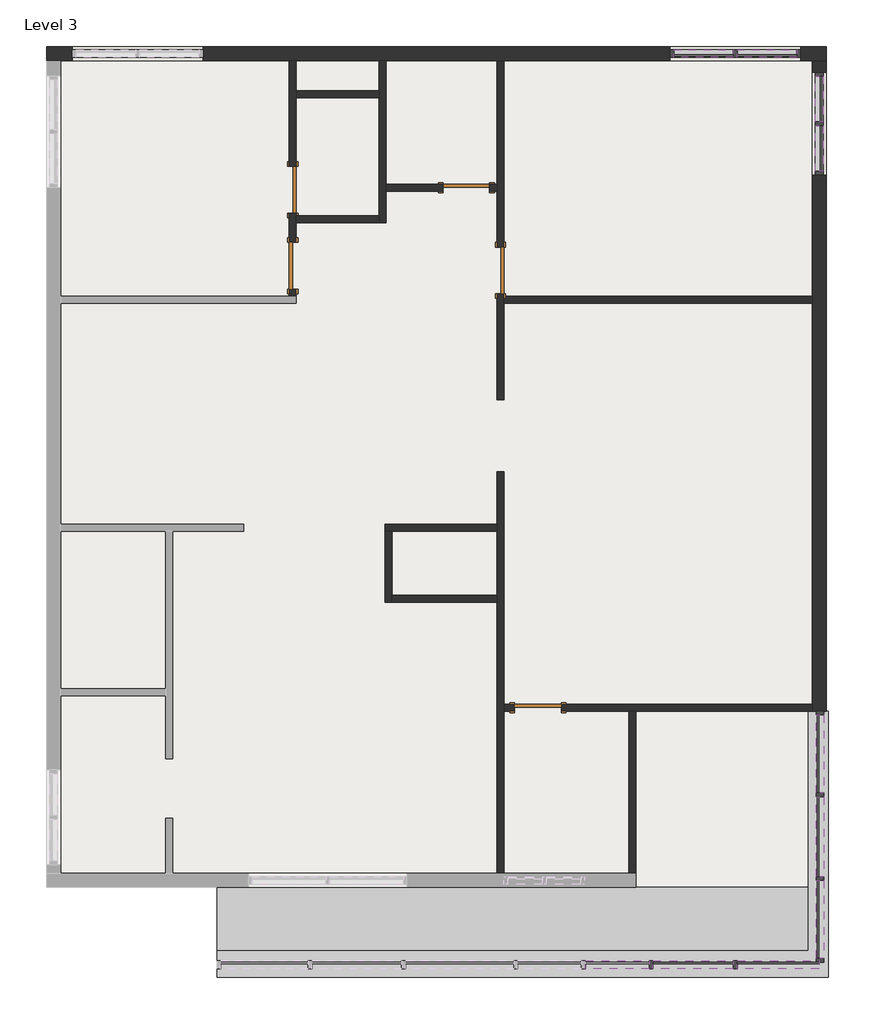
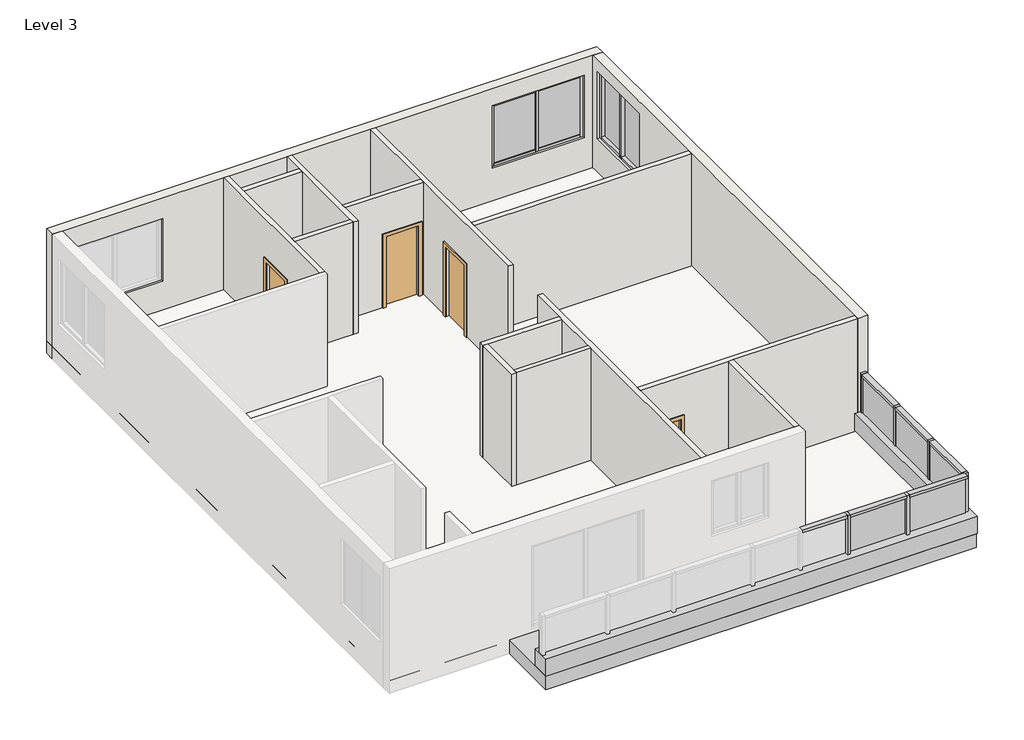
# One storey, part 2 of 2: 26 members, 15 walls, 9 plates, 5 doors, 1 proxy, 1 roof.
"""IFC4 building model written with IfcOpenShell, lengths in millimetres."""

from ifc_helpers import new_model, si_unit, frame, origin, place, context, project, spatial, polyline, outline, extrude, faceted_brep, transform, mapped, element, save
from components import generic_models_5_generic_models_5_36a2ceba, door_f2b275c1, door_d8f5dbb5, member_3a0a7659, member_801a2072, member_0bc49b9d, member_ce46b7cd, member_bcb10b1d, member_032a0f9a, member_dda01c07, member_04769ced, member_d37749d9, member_69204bcc, member_aead4eab, member_d6537dc6, member_1988c634, member_477baa08, system_panel_glazed_822919b4, system_panel_glazed_5228c6df, system_panel_glazed_6547e81a, system_panel_glazed_b56c0438, system_panel_glazed_688ed8e9, system_panel_glazed_5ee7ee01

model = new_model("IFC4")

# Units and contexts
model_context = context("Model", 3, world=origin())
ifc_project = project(units=[si_unit("LENGTHUNIT", "METRE", prefix="MILLI")], contexts=[model_context])

# Site, building, storey
site = spatial("IfcSite", under=ifc_project)
building = spatial("IfcBuilding", under=site)
storey = spatial("IfcBuildingStorey", under=building, Name="Level 3", Elevation=6096.0)

# Proxy
placement = place(None, origin())
generic_models_5_generic_models_5_shape = generic_models_5_generic_models_5_36a2ceba(model_context)
element("IfcBuildingElementProxy", 1, Name="Generic Models 5 : Generic Models 5", ObjectType="Generic Models 5 : Generic Models 5", at=placement, inside=storey, context=model_context, shape_type="MappedRepresentation", body=[
    mapped(generic_models_5_generic_models_5_shape, transform((0.0, 0.0, 0.0), x_axis=(1.0, 0.0, 0.0), y_axis=(0.0, 1.0, 0.0), z_axis=(0.0, 0.0, 1.0))),
])

# Doors
door_shape = door_f2b275c1(model_context)
element("IfcDoor", 2, ObjectType="Single-Flush : 30\" x 80\"", at=placement, inside=storey, context=model_context, shape_type="MappedRepresentation", body=[
    mapped(door_shape, transform((-14978.0695233, -3993.8252569, 6096.0), x_axis=(0.0, -1.0, 0.0), y_axis=(1.0, 0.0, 0.0), z_axis=(0.0, 0.0, 1.0))),
])
element("IfcDoor", 3, ObjectType="Single-Flush : 30\" x 80\"", at=placement, inside=storey, context=model_context, shape_type="MappedRepresentation", body=[
    mapped(door_shape, transform((-10977.5695233, -11201.0752569, 6096.0), x_axis=(-1.0, 0.0, 0.0), y_axis=(0.0, -1.0, 0.0), z_axis=(0.0, 0.0, 1.0))),
])
door_2_shape = door_d8f5dbb5(model_context)
element("IfcDoor", 4, ObjectType="Single-Flush : 30\" x 80\"", at=placement, inside=storey, context=model_context, shape_type="MappedRepresentation", body=[
    mapped(door_2_shape, transform((-14978.0695233, -2755.5752569, 6096.0), x_axis=(0.0, -1.0, 0.0), y_axis=(1.0, 0.0, 0.0), z_axis=(0.0, 0.0, 1.0))),
])
element("IfcDoor", 5, ObjectType="Single-Flush : 30\" x 80\"", at=placement, inside=storey, context=model_context, shape_type="MappedRepresentation", body=[
    mapped(door_2_shape, transform((-12145.9695233, -2723.8252569, 6096.0), x_axis=(1.0, 0.0, 0.0), y_axis=(0.0, 1.0, 0.0), z_axis=(0.0, 0.0, 1.0))),
])
element("IfcDoor", 6, ObjectType="Single-Flush : 30\" x 80\"", at=placement, inside=storey, context=model_context, shape_type="MappedRepresentation", body=[
    mapped(door_2_shape, transform((-11587.1695233, -4070.0252569, 6096.0), x_axis=(0.0, -1.0, 0.0), y_axis=(1.0, 0.0, 0.0), z_axis=(0.0, 0.0, 1.0))),
])

# Members
member_shape = member_3a0a7659(model_context)
element("IfcMember", 7, ObjectType="Rectangular Mullion : 2.5\" x 5\" rectangular", at=placement, inside=storey, context=model_context, shape_type="MappedRepresentation", body=[
    mapped(member_shape, transform((-6386.5195233, -1644.3252569, 8857.8668559), x_axis=(0.0, 0.0, 1.0), y_axis=(-1.0, 0.0, 0.0), z_axis=(0.0, -1.0, 0.0))),
])
element("IfcMember", 8, ObjectType="Rectangular Mullion : 2.5\" x 5\" rectangular", at=placement, inside=storey, context=model_context, shape_type="MappedRepresentation", body=[
    mapped(member_shape, transform((-6386.5195233, -2450.7752569, 8857.8668559), x_axis=(0.0, 0.0, 1.0), y_axis=(-1.0, 0.0, 0.0), z_axis=(0.0, -1.0, 0.0))),
])
element("IfcMember", 9, ObjectType="Rectangular Mullion : 2.5\" x 5\" rectangular", at=placement, inside=storey, context=model_context, shape_type="MappedRepresentation", body=[
    mapped(member_shape, transform((-6386.5195233, -1707.8252569, 7223.9300621), x_axis=(0.0, 0.0, -1.0), y_axis=(-1.0, 0.0, 0.0), z_axis=(0.0, 1.0, 0.0))),
])
element("IfcMember", 10, ObjectType="Rectangular Mullion : 2.5\" x 5\" rectangular", at=placement, inside=storey, context=model_context, shape_type="MappedRepresentation", body=[
    mapped(member_shape, transform((-6386.5195233, -901.3752569, 7223.9300621), x_axis=(0.0, 0.0, -1.0), y_axis=(-1.0, 0.0, 0.0), z_axis=(0.0, 1.0, 0.0))),
])
member_2_shape = member_801a2072(model_context)
element("IfcMember", 11, ObjectType="Rectangular Mullion : 2.5\" x 5\" rectangular", at=placement, inside=storey, context=model_context, shape_type="MappedRepresentation", body=[
    mapped(member_2_shape, transform((-8761.4195233, -533.0752569, 8728.0505251), x_axis=(0.0, 0.0, 1.0), y_axis=(0.0, 1.0, 0.0), z_axis=(-1.0, 0.0, 0.0))),
])
element("IfcMember", 12, ObjectType="Rectangular Mullion : 2.5\" x 5\" rectangular", at=placement, inside=storey, context=model_context, shape_type="MappedRepresentation", body=[
    mapped(member_2_shape, transform((-7726.3695233, -533.0752569, 8728.0505251), x_axis=(0.0, 0.0, 1.0), y_axis=(0.0, 1.0, 0.0), z_axis=(-1.0, 0.0, 0.0))),
])
element("IfcMember", 13, ObjectType="Rectangular Mullion : 2.5\" x 5\" rectangular", at=placement, inside=storey, context=model_context, shape_type="MappedRepresentation", body=[
    mapped(member_2_shape, transform((-6754.8195233, -533.0752569, 7198.162091), x_axis=(0.0, 0.0, -1.0), y_axis=(0.0, 1.0, 0.0), z_axis=(1.0, 0.0, 0.0))),
])
element("IfcMember", 14, ObjectType="Rectangular Mullion : 2.5\" x 5\" rectangular", at=placement, inside=storey, context=model_context, shape_type="MappedRepresentation", body=[
    mapped(member_2_shape, transform((-7789.8695233, -533.0752569, 7198.162091), x_axis=(0.0, 0.0, -1.0), y_axis=(0.0, 1.0, 0.0), z_axis=(1.0, 0.0, 0.0))),
])
member_3_shape = member_0bc49b9d(model_context)
element("IfcMember", 15, ObjectType="Rectangular Mullion : 2.5\" x 5\" rectangular", at=placement, inside=storey, context=model_context, shape_type="MappedRepresentation", body=[
    mapped(member_3_shape, transform((-6386.5195233, -1676.0752569, 7223.9300621), x_axis=(0.0, -1.0, 0.0), y_axis=(-1.0, 0.0, 0.0), z_axis=(0.0, 0.0, -1.0))),
])
member_4_shape = member_ce46b7cd(model_context)
element("IfcMember", 16, ObjectType="Rectangular Mullion : 2.5\" x 5\" rectangular", at=placement, inside=storey, context=model_context, shape_type="MappedRepresentation", body=[
    mapped(member_4_shape, transform((-6386.5195233, -837.8752569, 8857.8668559), x_axis=(0.0, 1.0, 0.0), y_axis=(-1.0, 0.0, 0.0), z_axis=(0.0, 0.0, 1.0))),
])
element("IfcMember", 17, ObjectType="Rectangular Mullion : 2.5\" x 5\" rectangular", at=placement, inside=storey, context=model_context, shape_type="MappedRepresentation", body=[
    mapped(member_4_shape, transform((-6386.5195233, -2514.2752569, 7223.9300621), x_axis=(0.0, -1.0, 0.0), y_axis=(-1.0, 0.0, 0.0), z_axis=(0.0, 0.0, -1.0))),
])
member_5_shape = member_bcb10b1d(model_context)
element("IfcMember", 18, ObjectType="Rectangular Mullion : 2.5\" x 5\" rectangular", at=placement, inside=storey, context=model_context, shape_type="MappedRepresentation", body=[
    mapped(member_5_shape, transform((-8824.9195233, -533.0752569, 7198.162091), x_axis=(-1.0, 0.0, 0.0), y_axis=(0.0, 1.0, 0.0), z_axis=(0.0, 0.0, -1.0))),
])
element("IfcMember", 19, ObjectType="Rectangular Mullion : 2.5\" x 5\" rectangular", at=placement, inside=storey, context=model_context, shape_type="MappedRepresentation", body=[
    mapped(member_5_shape, transform((-6691.3195233, -533.0752569, 8728.0505251), x_axis=(1.0, 0.0, 0.0), y_axis=(0.0, 1.0, 0.0), z_axis=(0.0, 0.0, 1.0))),
])
member_6_shape = member_032a0f9a(model_context)
element("IfcMember", 20, ObjectType="Rectangular Mullion : 2.5\" x 5\" rectangular", at=placement, inside=storey, context=model_context, shape_type="MappedRepresentation", body=[
    mapped(member_6_shape, transform((-7758.1195233, -533.0752569, 7198.162091), x_axis=(-1.0, 0.0, 0.0), y_axis=(0.0, 1.0, 0.0), z_axis=(0.0, 0.0, -1.0))),
])
member_7_shape = member_dda01c07(model_context)
element("IfcMember", 21, ObjectType="Rectangular Mullion : 2.5\" x 5\" rectangular", at=placement, inside=storey, context=model_context, shape_type="MappedRepresentation", body=[
    mapped(member_7_shape, transform((-9129.7195233, -15398.1130528, 6841.9204311), x_axis=(1.0, 0.0, 0.0), y_axis=(0.0, -1.0, 0.0), z_axis=(0.0, 0.0, -1.0))),
])
element("IfcMember", 22, ObjectType="Rectangular Mullion : 2.5\" x 5\" rectangular", at=placement, inside=storey, context=model_context, shape_type="MappedRepresentation", body=[
    mapped(member_7_shape, transform((-7758.1195233, -15398.1130528, 6841.9204311), x_axis=(1.0, 0.0, 0.0), y_axis=(0.0, -1.0, 0.0), z_axis=(0.0, 0.0, -1.0))),
])
member_8_shape = member_04769ced(model_context)
element("IfcMember", 23, ObjectType="Rectangular Mullion : 2.5\" x 5\" rectangular", at=placement, inside=storey, context=model_context, shape_type="MappedRepresentation", body=[
    mapped(member_8_shape, transform((-9161.4695233, -15398.1130528, 7802.9269124), x_axis=(0.0, 0.0, 1.0), y_axis=(0.0, -1.0, 0.0), z_axis=(1.0, 0.0, 0.0))),
])
member_9_shape = member_d37749d9(model_context)
element("IfcMember", 24, ObjectType="Rectangular Mullion : 2.5\" x 5\" rectangular", at=placement, inside=storey, context=model_context, shape_type="MappedRepresentation", body=[
    mapped(member_9_shape, transform((-7789.8695233, -15398.1130528, 7802.9269124), x_axis=(0.0, 0.0, 1.0), y_axis=(0.0, -1.0, 0.0), z_axis=(1.0, 0.0, 0.0))),
])
member_10_shape = member_69204bcc(model_context)
element("IfcMember", 25, ObjectType="Rectangular Mullion : 2.5\" x 5\" rectangular", at=placement, inside=storey, context=model_context, shape_type="MappedRepresentation", body=[
    mapped(member_10_shape, transform((-6386.5195233, -15398.1130528, 7802.9269124), x_axis=(0.0, 0.0, 1.0), y_axis=(0.0, -1.0, 0.0), z_axis=(1.0, 0.0, 0.0))),
])
member_11_shape = member_aead4eab(model_context)
element("IfcMember", 26, ObjectType="Rectangular Mullion : 2.5\" x 5\" rectangular", at=placement, inside=storey, context=model_context, shape_type="MappedRepresentation", body=[
    mapped(member_11_shape, transform((-6374.7212454, -15353.6630528, 7790.2317703), x_axis=(0.0, -1.0, 0.0), y_axis=(1.0, 0.0, 0.0), z_axis=(0.0, 0.0, 1.0))),
])
member_12_shape = member_d6537dc6(model_context)
element("IfcMember", 27, ObjectType="Rectangular Mullion : 2.5\" x 5\" rectangular", at=placement, inside=storey, context=model_context, shape_type="MappedRepresentation", body=[
    mapped(member_12_shape, transform((-6374.7212454, -14020.2671209, 7790.2317703), x_axis=(0.0, 0.0, 1.0), y_axis=(1.0, 0.0, 0.0), z_axis=(0.0, 1.0, 0.0))),
])
element("IfcMember", 28, ObjectType="Rectangular Mullion : 2.5\" x 5\" rectangular", at=placement, inside=storey, context=model_context, shape_type="MappedRepresentation", body=[
    mapped(member_12_shape, transform((-6374.7212454, -11321.7252569, 7790.2317703), x_axis=(0.0, 0.0, 1.0), y_axis=(1.0, 0.0, 0.0), z_axis=(0.0, 1.0, 0.0))),
])
member_13_shape = member_1988c634(model_context)
element("IfcMember", 29, ObjectType="Rectangular Mullion : 2.5\" x 5\" rectangular", at=placement, inside=storey, context=model_context, shape_type="MappedRepresentation", body=[
    mapped(member_13_shape, transform((-6374.7212454, -13988.5171209, 6841.9204311), x_axis=(0.0, 1.0, 0.0), y_axis=(1.0, 0.0, 0.0), z_axis=(0.0, 0.0, -1.0))),
])
element("IfcMember", 30, ObjectType="Rectangular Mullion : 2.5\" x 5\" rectangular", at=placement, inside=storey, context=model_context, shape_type="MappedRepresentation", body=[
    mapped(member_13_shape, transform((-6374.7212454, -12623.3711889, 6841.9204311), x_axis=(0.0, 1.0, 0.0), y_axis=(1.0, 0.0, 0.0), z_axis=(0.0, 0.0, -1.0))),
])
member_14_shape = member_477baa08(model_context)
element("IfcMember", 31, ObjectType="Rectangular Mullion : 2.5\" x 5\" rectangular", at=placement, inside=storey, context=model_context, shape_type="MappedRepresentation", body=[
    mapped(member_14_shape, transform((-6374.7212454, -12655.1211889, 7790.2317703), x_axis=(0.0, 0.0, 1.0), y_axis=(1.0, 0.0, 0.0), z_axis=(0.0, 1.0, 0.0))),
])
element("IfcMember", 32, ObjectType="Rectangular Mullion : 2.5\" x 5\" rectangular", at=placement, inside=storey, context=model_context, shape_type="MappedRepresentation", body=[
    mapped(member_11_shape, transform((-6374.7212454, -11258.2252569, 6841.9204311), x_axis=(0.0, 1.0, 0.0), y_axis=(1.0, 0.0, 0.0), z_axis=(0.0, 0.0, -1.0))),
])

# Plates
system_panel_glazed_shape = system_panel_glazed_822919b4(model_context)
element("IfcPlate", 33, ObjectType="System Panel : Glazed", at=placement, inside=storey, context=model_context, shape_type="MappedRepresentation", body=[
    mapped(system_panel_glazed_shape, transform((-6386.5195233, -1272.8502569, 7287.4300621), x_axis=(0.0, -1.0, 0.0), y_axis=(1.0, 0.0, 0.0), z_axis=(0.0, 0.0, 1.0))),
])
element("IfcPlate", 34, ObjectType="System Panel : Glazed", at=placement, inside=storey, context=model_context, shape_type="MappedRepresentation", body=[
    mapped(system_panel_glazed_shape, transform((-6386.5195233, -2079.3002569, 7287.4300621), x_axis=(0.0, -1.0, 0.0), y_axis=(1.0, 0.0, 0.0), z_axis=(0.0, 0.0, 1.0))),
])
system_panel_glazed_2_shape = system_panel_glazed_5228c6df(model_context)
element("IfcPlate", 35, ObjectType="System Panel : Glazed", at=placement, inside=storey, context=model_context, shape_type="MappedRepresentation", body=[
    mapped(system_panel_glazed_2_shape, transform((-7240.5945233, -533.0752569, 7261.662091), x_axis=(-1.0, 0.0, 0.0), y_axis=(0.0, -1.0, 0.0), z_axis=(0.0, 0.0, 1.0))),
])
element("IfcPlate", 36, ObjectType="System Panel : Glazed", at=placement, inside=storey, context=model_context, shape_type="MappedRepresentation", body=[
    mapped(system_panel_glazed_2_shape, transform((-8275.6445233, -533.0752569, 7261.662091), x_axis=(-1.0, 0.0, 0.0), y_axis=(0.0, -1.0, 0.0), z_axis=(0.0, 0.0, 1.0))),
])
system_panel_glazed_3_shape = system_panel_glazed_6547e81a(model_context)
element("IfcPlate", 37, ObjectType="System Panel : Glazed", at=placement, inside=storey, context=model_context, shape_type="MappedRepresentation", body=[
    mapped(system_panel_glazed_3_shape, transform((-7056.4445233, -15398.1130528, 6841.9204311), x_axis=(1.0, 0.0, 0.0), y_axis=(0.0, 1.0, 0.0), z_axis=(0.0, 0.0, 1.0))),
])
system_panel_glazed_4_shape = system_panel_glazed_b56c0438(model_context)
element("IfcPlate", 38, ObjectType="System Panel : Glazed", at=placement, inside=storey, context=model_context, shape_type="MappedRepresentation", body=[
    mapped(system_panel_glazed_4_shape, transform((-8443.9195233, -15398.1130528, 6841.9204311), x_axis=(1.0, 0.0, 0.0), y_axis=(0.0, 1.0, 0.0), z_axis=(0.0, 0.0, 1.0))),
])
system_panel_glazed_5_shape = system_panel_glazed_688ed8e9(model_context)
element("IfcPlate", 39, ObjectType="System Panel : Glazed", at=placement, inside=storey, context=model_context, shape_type="MappedRepresentation", body=[
    mapped(system_panel_glazed_5_shape, transform((-6374.7212454, -14655.2150868, 6841.9204311), x_axis=(0.0, 1.0, 0.0), y_axis=(-1.0, 0.0, 0.0), z_axis=(0.0, 0.0, 1.0))),
])
element("IfcPlate", 40, ObjectType="System Panel : Glazed", at=placement, inside=storey, context=model_context, shape_type="MappedRepresentation", body=[
    mapped(system_panel_glazed_5_shape, transform((-6374.7212454, -11956.6732229, 6841.9204311), x_axis=(0.0, 1.0, 0.0), y_axis=(-1.0, 0.0, 0.0), z_axis=(0.0, 0.0, 1.0))),
])
system_panel_glazed_6_shape = system_panel_glazed_5ee7ee01(model_context)
element("IfcPlate", 41, ObjectType="System Panel : Glazed", at=placement, inside=storey, context=model_context, shape_type="MappedRepresentation", body=[
    mapped(system_panel_glazed_6_shape, transform((-6374.7212454, -13305.9441549, 6841.9204311), x_axis=(0.0, 1.0, 0.0), y_axis=(-1.0, 0.0, 0.0), z_axis=(0.0, 0.0, 1.0))),
])

# Roof
element("IfcRoof", 42, ObjectType="Generic - 12\"", at=placement, inside=storey, context=model_context, shape_type="SweptSolid", body=[
    extrude(outline(polyline([(-18997.6195233, -418.7752569), (-6272.2195233, -418.7752569), (-6272.2195233, -14134.7752569), (-18997.6195233, -14134.7752569), (-18997.6195233, -418.7752569)])), frame((0.0, 0.0, 6096.0), z_axis=(0.0, 0.0, 1.0), x_axis=(1.0, 0.0, 0.0)), (0.0, 0.0, 1.0), 304.8),
])

# Walls
element("IfcWall", 43, ObjectType="4.5\"", at=placement, inside=storey, context=model_context, shape_type="Brep", body=[
    faceted_brep([(-14920.9195233, -3612.8252569, 6096.0), (-14920.9195233, -3295.3252569, 6096.0), (-14920.9195233, -3181.0252569, 6096.0), (-14920.9195233, -3136.5752569, 6096.0), (-14920.9195233, -3136.5752569, 8128.0), (-14920.9195233, -2374.5752569, 8128.0), (-14920.9195233, -2374.5752569, 6096.0), (-14920.9195233, -1256.9752569, 6096.0), (-14920.9195233, -1142.6752569, 6096.0), (-14920.9195233, -647.3752569, 6096.0), (-14920.9195233, -647.3752569, 9144.0), (-14920.9195233, -1142.6752569, 9144.0), (-14920.9195233, -1256.9752569, 9144.0), (-14920.9195233, -3181.0252569, 9144.0), (-14920.9195233, -3295.3252569, 9144.0), (-14920.9195233, -4495.4752569, 9144.0), (-14920.9195233, -4495.4752569, 6096.0), (-14920.9195233, -4374.8252569, 6096.0), (-14920.9195233, -4374.8252569, 8128.0), (-14920.9195233, -3612.8252569, 8128.0), (-15035.2195233, -3136.5752569, 8128.0), (-15035.2195233, -3136.5752569, 6096.0), (-15035.2195233, -3612.8252569, 6096.0), (-15035.2195233, -3612.8252569, 8128.0), (-15035.2195233, -4374.8252569, 8128.0), (-15035.2195233, -4374.8252569, 6096.0), (-15035.2195233, -4495.4752569, 6096.0), (-15035.2195233, -4495.4752569, 9144.0), (-15035.2195233, -647.3752569, 9144.0), (-15035.2195233, -647.3752569, 6096.0), (-15035.2195233, -2374.5752569, 6096.0), (-15035.2195233, -2374.5752569, 8128.0)], [[[0, 1, 2, 3, 4, 5, 6, 7, 8, 9, 10, 11, 12, 13, 14, 15, 16, 17, 18, 19]], [[20, 21, 22, 23, 24, 25, 26, 27, 28, 29, 30, 31]], [[26, 25, 17, 16]], [[30, 29, 9, 8, 7, 6]], [[22, 21, 3, 2, 1, 0]], [[15, 14, 13, 12, 11, 10, 28, 27]], [[16, 15, 27, 26]], [[10, 9, 29, 28]], [[18, 17, 25, 24]], [[19, 18, 24, 23]], [[0, 19, 23, 22]], [[4, 3, 21, 20]], [[5, 4, 20, 31]], [[6, 5, 31, 30]]]),
])
element("IfcWall", 44, ObjectType="4.5\"", at=placement, inside=storey, context=model_context, shape_type="SweptSolid", body=[
    extrude(outline(polyline([(-13568.3695233, -1256.9752569), (-14920.9195233, -1256.9752569), (-14920.9195233, -1142.6752569), (-13568.3695233, -1142.6752569), (-13568.3695233, -1256.9752569)])), frame((0.0, 0.0, 6096.0), z_axis=(0.0, 0.0, 1.0), x_axis=(1.0, 0.0, 0.0)), (0.0, 0.0, 1.0), 3048.0),
])
element("IfcWall", 45, ObjectType="4.5\"", at=placement, inside=storey, context=model_context, shape_type="Brep", body=[
    faceted_brep([(-13454.0695233, -3295.3252569, 6096.0), (-13454.0695233, -2780.9752569, 6096.0), (-13454.0695233, -2666.6752569, 6096.0), (-13454.0695233, -647.3752569, 6096.0), (-13454.0695233, -647.3752569, 9144.0), (-13454.0695233, -2666.6752569, 9144.0), (-13454.0695233, -2780.9752569, 9144.0), (-13454.0695233, -3295.3252569, 9144.0), (-13568.3695233, -3295.3252569, 6096.0), (-13568.3695233, -3295.3252569, 9144.0), (-13568.3695233, -3181.0252569, 9144.0), (-13568.3695233, -1256.9752569, 9144.0), (-13568.3695233, -1142.6752569, 9144.0), (-13568.3695233, -647.3752569, 9144.0), (-13568.3695233, -647.3752569, 6096.0), (-13568.3695233, -1142.6752569, 6096.0), (-13568.3695233, -1256.9752569, 6096.0), (-13568.3695233, -3181.0252569, 6096.0)], [[[0, 1, 2, 3, 4, 5, 6, 7]], [[8, 9, 10, 11, 12, 13, 14, 15, 16, 17]], [[3, 2, 1, 0, 8, 17, 16, 15, 14]], [[7, 6, 5, 4, 13, 12, 11, 10, 9]], [[4, 3, 14, 13]], [[0, 7, 9, 8]]]),
])
element("IfcWall", 46, ObjectType="4.5\"", at=placement, inside=storey, context=model_context, shape_type="SweptSolid", body=[
    extrude(outline(polyline([(-14920.9195233, -3181.0252569), (-13568.3695233, -3181.0252569), (-13568.3695233, -3295.3252569), (-14920.9195233, -3295.3252569), (-14920.9195233, -3181.0252569)])), frame((0.0, 0.0, 6096.0), z_axis=(0.0, 0.0, 1.0), x_axis=(1.0, 0.0, 0.0)), (0.0, 0.0, 1.0), 3048.0),
])
element("IfcWall", 47, ObjectType="4.5\"", at=placement, inside=storey, context=model_context, shape_type="SweptSolid", body=[
    extrude(outline(polyline([(8128.0, -11764.9695233), (6096.0, -11764.9695233), (6096.0, -11644.3195233), (9144.0, -11644.3195233), (9144.0, -13454.0695233), (6096.0, -13454.0695233), (6096.0, -12526.9695233), (8128.0, -12526.9695233), (8128.0, -11764.9695233)])), frame((0.0, -2780.9752569, 0.0), z_axis=(0.0, 1.0, 0.0), x_axis=(0.0, 0.0, 1.0)), (0.0, 0.0, 1.0), 114.3),
])
element("IfcWall", 48, ObjectType="4.5\"", at=placement, inside=storey, context=model_context, shape_type="Brep", body=[
    faceted_brep([(-11644.3195233, -4451.0252569, 8128.0), (-11644.3195233, -4451.0252569, 6096.0), (-11644.3195233, -6178.2252569, 6096.0), (-11644.3195233, -6178.2252569, 9144.0), (-11644.3195233, -2780.9752569, 9144.0), (-11644.3195233, -2666.6752569, 9144.0), (-11644.3195233, -647.3752569, 9144.0), (-11644.3195233, -647.3752569, 6096.0), (-11644.3195233, -2666.6752569, 6096.0), (-11644.3195233, -2780.9752569, 6096.0), (-11644.3195233, -3689.0252569, 6096.0), (-11644.3195233, -3689.0252569, 8128.0), (-11530.0195233, -6178.2252569, 6096.0), (-11530.0195233, -4609.7752569, 6096.0), (-11530.0195233, -4495.4752569, 6096.0), (-11530.0195233, -4451.0252569, 6096.0), (-11530.0195233, -4451.0252569, 8128.0), (-11530.0195233, -3689.0252569, 8128.0), (-11530.0195233, -3689.0252569, 6096.0), (-11530.0195233, -647.3752569, 6096.0), (-11530.0195233, -647.3752569, 9144.0), (-11530.0195233, -4495.4752569, 9144.0), (-11530.0195233, -4609.7752569, 9144.0), (-11530.0195233, -6178.2252569, 9144.0)], [[[0, 1, 2, 3, 4, 5, 6, 7, 8, 9, 10, 11]], [[12, 13, 14, 15, 16, 17, 18, 19, 20, 21, 22, 23]], [[2, 1, 15, 14, 13, 12]], [[10, 9, 8, 7, 19, 18]], [[3, 2, 12, 23]], [[6, 5, 4, 3, 23, 22, 21, 20]], [[7, 6, 20, 19]], [[16, 15, 1, 0]], [[17, 16, 0, 11]], [[18, 17, 11, 10]]]),
])
element("IfcWall", 49, ObjectType="4.5\"", at=placement, inside=storey, context=model_context, shape_type="SweptSolid", body=[
    extrude(outline(polyline([(-6500.8195233, -4609.7752569), (-11530.0195233, -4609.7752569), (-11530.0195233, -4495.4752569), (-6500.8195233, -4495.4752569), (-6500.8195233, -4609.7752569)])), frame((0.0, 0.0, 6096.0), z_axis=(0.0, 0.0, 1.0), x_axis=(1.0, 0.0, 0.0)), (0.0, 0.0, 1.0), 3048.0),
])
element("IfcWall", 50, ObjectType="4.5\"", at=placement, inside=storey, context=model_context, shape_type="Brep", body=[
    faceted_brep([(-11530.0195233, -13906.1752569, 6096.0), (-11530.0195233, -11258.2252569, 6096.0), (-11530.0195233, -11143.9252569, 6096.0), (-11530.0195233, -7352.9752569, 6096.0), (-11530.0195233, -7352.9752569, 9144.0), (-11530.0195233, -11143.9252569, 9144.0), (-11530.0195233, -11258.2252569, 9144.0), (-11530.0195233, -13906.1752569, 9144.0), (-11644.3195233, -13906.1752569, 6096.0), (-11644.3195233, -13906.1752569, 9144.0), (-11644.3195233, -9486.5752569, 9144.0), (-11644.3195233, -9372.2752569, 9144.0), (-11644.3195233, -8324.5252569, 9144.0), (-11644.3195233, -8210.2252569, 9144.0), (-11644.3195233, -7352.9752569, 9144.0), (-11644.3195233, -7352.9752569, 6096.0), (-11644.3195233, -8210.2252569, 6096.0), (-11644.3195233, -8324.5252569, 6096.0), (-11644.3195233, -9372.2752569, 6096.0), (-11644.3195233, -9486.5752569, 6096.0)], [[[0, 1, 2, 3, 4, 5, 6, 7]], [[8, 9, 10, 11, 12, 13, 14, 15, 16, 17, 18, 19]], [[3, 2, 1, 0, 8, 19, 18, 17, 16, 15]], [[4, 3, 15, 14]], [[7, 6, 5, 4, 14, 13, 12, 11, 10, 9]], [[0, 7, 9, 8]]]),
])
element("IfcWall", 51, ObjectType="4.5\"", at=placement, inside=storey, context=model_context, shape_type="Brep", body=[
    faceted_brep([(-13473.1195233, -8324.5252569, 6096.0), (-13358.8195233, -8324.5252569, 6096.0), (-11644.3195233, -8324.5252569, 6096.0), (-11644.3195233, -8324.5252569, 9144.0), (-13358.8195233, -8324.5252569, 9144.0), (-13473.1195233, -8324.5252569, 9144.0), (-13473.1195233, -8210.2252569, 6096.0), (-13473.1195233, -8210.2252569, 9144.0), (-11644.3195233, -8210.2252569, 9144.0), (-11644.3195233, -8210.2252569, 6096.0)], [[[0, 1, 2, 3, 4, 5]], [[6, 7, 8, 9]], [[2, 1, 0, 6, 9]], [[5, 4, 3, 8, 7]], [[3, 2, 9, 8]], [[0, 5, 7, 6]]]),
])
element("IfcWall", 52, ObjectType="4.5\"", at=placement, inside=storey, context=model_context, shape_type="Brep", body=[
    faceted_brep([(-13473.1195233, -8324.5252569, 6096.0), (-13473.1195233, -9486.5752569, 6096.0), (-13473.1195233, -9486.5752569, 9144.0), (-13473.1195233, -8324.5252569, 9144.0), (-13358.8195233, -8324.5252569, 6096.0), (-13358.8195233, -8324.5252569, 9144.0), (-13358.8195233, -9372.2752569, 9144.0), (-13358.8195233, -9486.5752569, 9144.0), (-13358.8195233, -9486.5752569, 6096.0), (-13358.8195233, -9372.2752569, 6096.0)], [[[0, 1, 2, 3]], [[4, 5, 6, 7, 8, 9]], [[1, 0, 4, 9, 8]], [[3, 2, 7, 6, 5]], [[0, 3, 5, 4]], [[2, 1, 8, 7]]]),
])
element("IfcWall", 53, ObjectType="4.5\"", at=placement, inside=storey, context=model_context, shape_type="SweptSolid", body=[
    extrude(outline(polyline([(-11644.3195233, -9486.5752569), (-13358.8195233, -9486.5752569), (-13358.8195233, -9372.2752569), (-11644.3195233, -9372.2752569), (-11644.3195233, -9486.5752569)])), frame((0.0, 0.0, 6096.0), z_axis=(0.0, 0.0, 1.0), x_axis=(1.0, 0.0, 0.0)), (0.0, 0.0, 1.0), 3048.0),
])
element("IfcWall", 54, ObjectType="4.5\"", at=placement, inside=storey, context=model_context, shape_type="Brep", body=[
    faceted_brep([(-11530.0195233, -11258.2252569, 6096.0), (-11358.5695233, -11258.2252569, 6096.0), (-11358.5695233, -11258.2252569, 8128.0), (-10596.5695233, -11258.2252569, 8128.0), (-10596.5695233, -11258.2252569, 6096.0), (-9491.6695233, -11258.2252569, 6096.0), (-9377.3695233, -11258.2252569, 6096.0), (-6500.8195233, -11258.2252569, 6096.0), (-6500.8195233, -11258.2252569, 9144.0), (-9377.3695233, -11258.2252569, 9144.0), (-9491.6695233, -11258.2252569, 9144.0), (-11530.0195233, -11258.2252569, 9144.0), (-11358.5695233, -11143.9252569, 8128.0), (-11358.5695233, -11143.9252569, 6096.0), (-11530.0195233, -11143.9252569, 6096.0), (-11530.0195233, -11143.9252569, 9144.0), (-6500.8195233, -11143.9252569, 9144.0), (-6500.8195233, -11143.9252569, 6096.0), (-10596.5695233, -11143.9252569, 6096.0), (-10596.5695233, -11143.9252569, 8128.0)], [[[0, 1, 2, 3, 4, 5, 6, 7, 8, 9, 10, 11]], [[12, 13, 14, 15, 16, 17, 18, 19]], [[18, 17, 7, 6, 5, 4]], [[14, 13, 1, 0]], [[11, 10, 9, 8, 16, 15]], [[8, 7, 17, 16]], [[0, 11, 15, 14]], [[2, 1, 13, 12]], [[3, 2, 12, 19]], [[4, 3, 19, 18]]]),
])
element("IfcWall", 55, ObjectType="4.5\"", at=placement, inside=storey, context=model_context, shape_type="SweptSolid", body=[
    extrude(outline(polyline([(-9491.6695233, -13906.1752569), (-9491.6695233, -11258.2252569), (-9377.3695233, -11258.2252569), (-9377.3695233, -13906.1752569), (-9491.6695233, -13906.1752569)])), frame((0.0, 0.0, 6096.0), z_axis=(0.0, 0.0, 1.0), x_axis=(1.0, 0.0, 0.0)), (0.0, 0.0, 1.0), 3048.0),
])
element("IfcWall", 56, ObjectType="9\"", at=placement, inside=storey, context=model_context, shape_type="Brep", body=[
    faceted_brep([(-18997.6195233, -647.3752569, 6096.0), (-18769.0195233, -647.3752569, 6096.0), (-15035.2195233, -647.3752569, 6096.0), (-14920.9195233, -647.3752569, 6096.0), (-13568.3695233, -647.3752569, 6096.0), (-13454.0695233, -647.3752569, 6096.0), (-11644.3195233, -647.3752569, 6096.0), (-11530.0195233, -647.3752569, 6096.0), (-6500.8195233, -647.3752569, 6096.0), (-6272.2195233, -647.3752569, 6096.0), (-6272.2195233, -647.3752569, 9144.0), (-6500.8195233, -647.3752569, 9144.0), (-11530.0195233, -647.3752569, 9144.0), (-11644.3195233, -647.3752569, 9144.0), (-13454.0695233, -647.3752569, 9144.0), (-13568.3695233, -647.3752569, 9144.0), (-14920.9195233, -647.3752569, 9144.0), (-15035.2195233, -647.3752569, 9144.0), (-18769.0195233, -647.3752569, 9144.0), (-18997.6195233, -647.3752569, 9144.0), (-6691.3195233, -647.3752569, 8728.0505251), (-6691.3195233, -647.3752569, 7198.162091), (-8824.9195233, -647.3752569, 7198.162091), (-8824.9195233, -647.3752569, 8728.0505251), (-18578.5195233, -647.3752569, 7102.6124164), (-18578.5195233, -647.3752569, 8635.8598955), (-16444.9195233, -647.3752569, 8635.8598955), (-16444.9195233, -647.3752569, 7102.6124164), (-6272.2195233, -418.7752569, 6096.0), (-18997.6195233, -418.7752569, 6096.0), (-18997.6195233, -418.7752569, 9144.0), (-6272.2195233, -418.7752569, 9144.0), (-6691.3195233, -418.7752569, 7198.162091), (-6691.3195233, -418.7752569, 8728.0505251), (-8824.9195233, -418.7752569, 8728.0505251), (-8824.9195233, -418.7752569, 7198.162091), (-18578.5195233, -418.7752569, 8635.8598955), (-18578.5195233, -418.7752569, 7102.6124164), (-16444.9195233, -418.7752569, 7102.6124164), (-16444.9195233, -418.7752569, 8635.8598955)], [[[0, 1, 2, 3, 4, 5, 6, 7, 8, 9, 10, 11, 12, 13, 14, 15, 16, 17, 18, 19], [20, 21, 22, 23], [24, 25, 26, 27]], [[28, 29, 30, 31], [32, 33, 34, 35], [36, 37, 38, 39]], [[9, 8, 7, 6, 5, 4, 3, 2, 1, 0, 29, 28]], [[19, 18, 17, 16, 15, 14, 13, 12, 11, 10, 31, 30]], [[10, 9, 28, 31]], [[0, 19, 30, 29]], [[20, 33, 32, 21]], [[33, 20, 23, 34]], [[34, 23, 22, 35]], [[21, 32, 35, 22]], [[24, 37, 36, 25]], [[25, 36, 39, 26]], [[26, 39, 38, 27]], [[37, 24, 27, 38]]]),
])
element("IfcWall", 57, ObjectType="9\"", at=placement, inside=storey, context=model_context, shape_type="Brep", body=[
    faceted_brep([(-6500.8195233, -647.3752569, 6096.0), (-6500.8195233, -4495.4752569, 6096.0), (-6500.8195233, -4609.7752569, 6096.0), (-6500.8195233, -11143.9252569, 6096.0), (-6500.8195233, -11258.2252569, 6096.0), (-6500.8195233, -11258.2252569, 9144.0), (-6500.8195233, -11143.9252569, 9144.0), (-6500.8195233, -4609.7752569, 9144.0), (-6500.8195233, -4495.4752569, 9144.0), (-6500.8195233, -647.3752569, 9144.0), (-6500.8195233, -837.8752569, 7223.9300621), (-6500.8195233, -837.8752569, 8857.8668559), (-6500.8195233, -2514.2752569, 8857.8668559), (-6500.8195233, -2514.2752569, 7223.9300621), (-6272.2195233, -11258.2252569, 6096.0), (-6272.2195233, -647.3752569, 6096.0), (-6272.2195233, -647.3752569, 9144.0), (-6272.2195233, -11258.2252569, 9144.0), (-6272.2195233, -837.8752569, 8857.8668559), (-6272.2195233, -837.8752569, 7223.9300621), (-6272.2195233, -2514.2752569, 7223.9300621), (-6272.2195233, -2514.2752569, 8857.8668559)], [[[0, 1, 2, 3, 4, 5, 6, 7, 8, 9], [10, 11, 12, 13]], [[14, 15, 16, 17], [18, 19, 20, 21]], [[4, 3, 2, 1, 0, 15, 14]], [[5, 4, 14, 17]], [[9, 8, 7, 6, 5, 17, 16]], [[0, 9, 16, 15]], [[10, 19, 18, 11]], [[11, 18, 21, 12]], [[12, 21, 20, 13]], [[19, 10, 13, 20]]]),
])

save(model, "model.ifc")

# Revit data of these elements
# Type "Single-Flush : 30\" x 80\""
#   Type Mark = "5"
#   Construction Type Id = "MDOOR"
#   Assembly Code = "C1020"
#   Analytic Construction = "Metal"
#   Thickness = 0' - 2"
#   Heat Transfer Coefficient (U) = 0.651978 BTU/(h·ft²·°F)
#   Height = 6' - 8"
#   Trim Projection Ext = 0' - 1"
#   Trim Projection Int = 0' - 1"
#   Trim Width = 0' - 3"
#   Width = 2' - 6"
#   Define Thermal Properties by = 1
#   Define Thermal Properties by = 1
#   Door Material = Door - Panel
#   Frame Material = Door - Frame
#   Visual Light Transmittance = 0
#   Solar Heat Gain Coefficient = 0
#   Function = (empty or 0)
#   Wall Closure = (empty or 0)
# Type "Rectangular Mullion : 2.5\" x 5\" rectangular"
#   built-in parameter 1007304 = 0.416667 (stored number, unit not read)
#   built-in parameter 1007301 = 0.104167 (stored number, unit not read)
#   built-in parameter 1007300 = 0.104167 (stored number, unit not read)
# Type "System Panel : Glazed"
#   Construction Type Id = "GSP4R"
#   Analytic Construction = "1/8 in Pilkington single glazing"
#   Visual Light Transmittance = 0.9
#   Solar Heat Gain Coefficient = 0.86
#   Heat Transfer Coefficient (U) = 1.18115 BTU/(h·ft²·°F)
#   Define Thermal Properties by = 1
# Type "Generic - 12\""
#   Assembly Code = "B1020"
#   Layers, outside or top first: 1' - 0" no material (function 1)
# Type "4.5\""
#   Assembly Code = "B2010"
#   Layers, outside or top first: 0' - 4 1/2" no material (function 1)
# Type "9\""
#   Assembly Code = "B2010"
#   Layers, outside or top first: 0' - 9" no material (function 1)
# Element 1 (IfcBuildingElementProxy, "Generic Models 5 : Generic Models 5")
#   Phase Created = New Construction
# Elements 2, 3, 4, 5, 6 (IfcDoor, "Single-Flush : 30\" x 80\"")
#   Phase Created = New Construction
#   Materials on its faces: "Door - Frame", "Door - Panel"
# Elements 7, 8, 9, 10, 11, 12, 13, 14, 15, 16, 17, 18, 19, 20, 21, 22, 23, 24, 25, 26, 27, 28, 29, 30, 31, 32 (IfcMember, "Rectangular Mullion : 2.5\" x 5\" rectangular")
#   Phase Created = New Construction
#   Materials on its faces: "Aluminum"
# Elements 33, 34, 35, 36, 37, 38, 39, 40, 41 (IfcPlate, "System Panel : Glazed")
#   Phase Created = New Construction
#   Materials on its faces: "Glass"
# Element 42 (IfcRoof, "Generic - 12\"")
#   built-in parameter 1001705 = 21 (stored number, unit not read)
#   built-in parameter 1001710 = 33615
#   Phase Created = New Construction
#   Materials on its faces: "Default Roof"
# Elements 43, 44, 45, 46, 47, 48, 49, 50, 51, 52, 53, 54, 55 (IfcWall, "4.5\"")
#   Top Offset = 0' - 0"
#   Base Offset = 0' - 0"
#   Unconnected Height = 10' - 0"
#   wall height = 10' - 0"
#   Phase Created = New Construction
#   Base Constraint = Level 3
#   Materials on its faces: "Default Wall"
# Elements 56, 57 (IfcWall, "9\"")
#   Top Offset = 0' - 0"
#   Base Offset = 0' - 0"
#   Unconnected Height = 10' - 0"
#   wall height = 10' - 0"
#   Phase Created = New Construction
#   Base Constraint = Level 3
#   Materials on its faces: "Default Wall"
# Materials
#   "Door - Panel": class "Wood", colour RGB 210 159 95, transparency 0, Cost = 0
#   "Door - Frame": colour RGB 118 70 51, transparency 0, Cost = 0
#   "Aluminum": class "Metal", colour RGB 247 247 247, transparency 0, Description = "Aluminum 6061", Cost = 0
#   "Glass": class "Glass", colour RGB 0 128 192, transparency 0.75, Description = "Soda Lime Glass", Cost = 0
#   "Default Roof": colour RGB 88 101 114, transparency 0, Cost = 0
#   "Default Wall": colour RGB 128 128 128, transparency 0, Cost = 0
